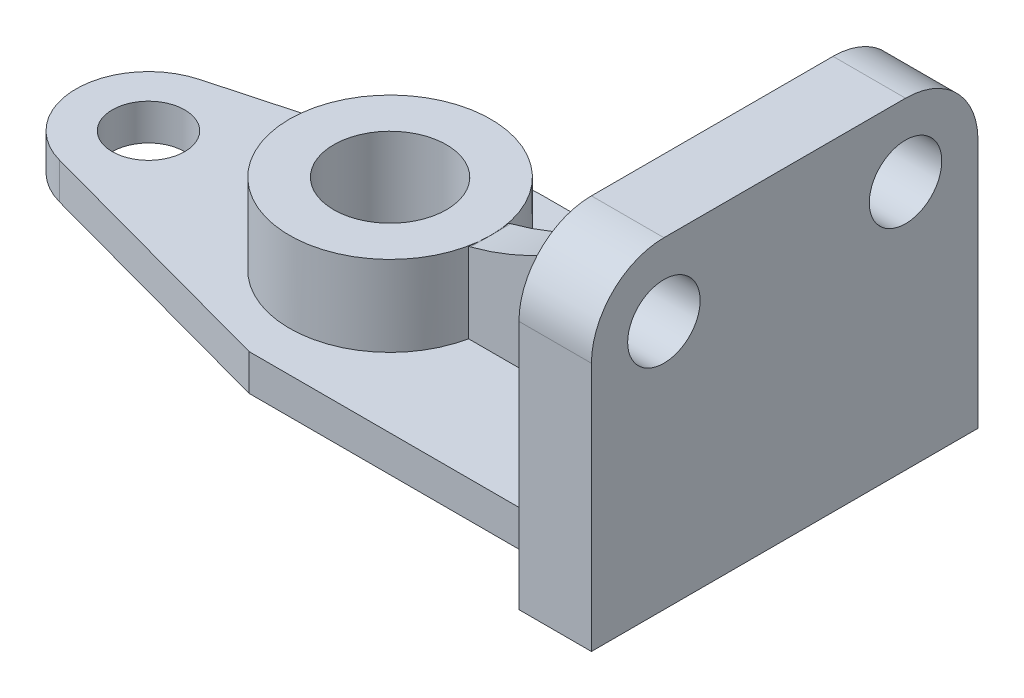
ISO-10303-21;
HEADER;
FILE_DESCRIPTION(('STEP AP214'),'2;1');
FILE_NAME('part.step','',(''),(''),'','','');
FILE_SCHEMA(('AUTOMOTIVE_DESIGN { 1 0 10303 214 1 1 1 1 }'));
ENDSEC;
DATA;
#1=APPLICATION_CONTEXT('core data for automotive mechanical design processes');
#2=APPLICATION_PROTOCOL_DEFINITION('international standard','automotive_design',2000,#1);
#3=PRODUCT_CONTEXT('',#1,'mechanical');
#4=PRODUCT('Part','Part','',(#3));
#5=PRODUCT_RELATED_PRODUCT_CATEGORY('part','',(#4));
#6=PRODUCT_DEFINITION_FORMATION('','',#4);
#7=PRODUCT_DEFINITION_CONTEXT('part definition',#1,'design');
#8=PRODUCT_DEFINITION('design','',#6,#7);
#9=PRODUCT_DEFINITION_SHAPE('','',#8);
#10=(LENGTH_UNIT() NAMED_UNIT(*) SI_UNIT(.MILLI.,.METRE.));
#11=(NAMED_UNIT(*) PLANE_ANGLE_UNIT() SI_UNIT($,.RADIAN.));
#12=(NAMED_UNIT(*) SI_UNIT($,.STERADIAN.) SOLID_ANGLE_UNIT());
#13=UNCERTAINTY_MEASURE_WITH_UNIT(LENGTH_MEASURE(1.E-05),#10,'distance_accuracy_value','');
#14=(GEOMETRIC_REPRESENTATION_CONTEXT(3) GLOBAL_UNCERTAINTY_ASSIGNED_CONTEXT((#13)) GLOBAL_UNIT_ASSIGNED_CONTEXT((#10,
#11,#12)) REPRESENTATION_CONTEXT('',''));
#15=CARTESIAN_POINT('',(0.,0.,0.));
#16=DIRECTION('',(0.,0.,1.));
#17=DIRECTION('',(1.,0.,0.));
#18=AXIS2_PLACEMENT_3D('',#15,#16,#17);
#19=CARTESIAN_POINT('',(-9.,-40.,48.));
#20=DIRECTION('',(1.,0.,0.));
#21=DIRECTION('',(0.,0.,-1.));
#22=AXIS2_PLACEMENT_3D('',#19,#20,#21);
#23=PLANE('',#22);
#24=CARTESIAN_POINT('',(-9.,22.,-30.));
#25=DIRECTION('',(-1.,0.,0.));
#26=DIRECTION('',(0.,0.,1.));
#27=AXIS2_PLACEMENT_3D('',#24,#25,#26);
#28=CIRCLE('',#27,9.);
#29=CARTESIAN_POINT('',(-9.,22.,-21.));
#30=VERTEX_POINT('',#29);
#31=EDGE_CURVE('E245',#30,#30,#28,.T.);
#32=ORIENTED_EDGE('',*,*,#31,.F.);
#33=EDGE_LOOP('',(#32));
#34=FACE_BOUND('',#33,.T.);
#35=DIRECTION('',(0.,-1.,0.));
#36=VECTOR('',#35,1.);
#37=CARTESIAN_POINT('',(-9.,-40.,-5.));
#38=LINE('',#37,#36);
#39=CARTESIAN_POINT('',(-9.,40.,-5.));
#40=VERTEX_POINT('',#39);
#41=CARTESIAN_POINT('',(-9.,-31.,-5.));
#42=VERTEX_POINT('',#41);
#43=EDGE_CURVE('E201',#40,#42,#38,.T.);
#44=ORIENTED_EDGE('',*,*,#43,.F.);
#45=DIRECTION('',(0.,0.,-1.));
#46=VECTOR('',#45,1.);
#47=CARTESIAN_POINT('',(-9.,40.,48.));
#48=LINE('',#47,#46);
#49=CARTESIAN_POINT('',(-9.,40.,-30.));
#50=VERTEX_POINT('',#49);
#51=EDGE_CURVE('E332',#40,#50,#48,.T.);
#52=ORIENTED_EDGE('',*,*,#51,.T.);
#53=CARTESIAN_POINT('',(-9.,22.,-30.));
#54=DIRECTION('',(1.,0.,0.));
#55=DIRECTION('',(0.,0.,-1.));
#56=AXIS2_PLACEMENT_3D('',#53,#54,#55);
#57=CIRCLE('',#56,18.);
#58=CARTESIAN_POINT('',(-9.,22.,-48.));
#59=VERTEX_POINT('',#58);
#60=EDGE_CURVE('E226',#50,#59,#57,.F.);
#61=ORIENTED_EDGE('',*,*,#60,.T.);
#62=DIRECTION('',(0.,-1.,0.));
#63=VECTOR('',#62,1.);
#64=CARTESIAN_POINT('',(-9.,-40.,-48.));
#65=LINE('',#64,#63);
#66=CARTESIAN_POINT('',(-9.,-31.,-48.));
#67=VERTEX_POINT('',#66);
#68=EDGE_CURVE('E326',#59,#67,#65,.T.);
#69=ORIENTED_EDGE('',*,*,#68,.T.);
#70=DIRECTION('',(0.,0.,1.));
#71=VECTOR('',#70,1.);
#72=CARTESIAN_POINT('',(-9.,-31.,-48.));
#73=LINE('',#72,#71);
#74=EDGE_CURVE('E311',#67,#42,#73,.T.);
#75=ORIENTED_EDGE('',*,*,#74,.T.);
#76=EDGE_LOOP('',(#44,#52,#61,#69,#75));
#77=FACE_BOUND('',#76,.T.);
#78=ADVANCED_FACE('F39',(#34,#77),#23,.F.);
#79=CARTESIAN_POINT('',(-9.,40.,48.));
#80=DIRECTION('',(0.,-1.,0.));
#81=DIRECTION('',(0.,0.,-1.));
#82=AXIS2_PLACEMENT_3D('',#79,#80,#81);
#83=PLANE('',#82);
#84=DIRECTION('',(0.,0.,-1.));
#85=VECTOR('',#84,1.);
#86=CARTESIAN_POINT('',(9.,40.,48.));
#87=LINE('',#86,#85);
#88=CARTESIAN_POINT('',(9.,40.,30.));
#89=VERTEX_POINT('',#88);
#90=CARTESIAN_POINT('',(9.,40.,-30.));
#91=VERTEX_POINT('',#90);
#92=EDGE_CURVE('E337',#89,#91,#87,.T.);
#93=ORIENTED_EDGE('',*,*,#92,.T.);
#94=DIRECTION('',(-1.,0.,0.));
#95=VECTOR('',#94,1.);
#96=CARTESIAN_POINT('',(9.,40.,-30.));
#97=LINE('',#96,#95);
#98=EDGE_CURVE('E231',#91,#50,#97,.T.);
#99=ORIENTED_EDGE('',*,*,#98,.T.);
#100=ORIENTED_EDGE('',*,*,#51,.F.);
#101=DIRECTION('',(0.,0.,1.));
#102=VECTOR('',#101,1.);
#103=CARTESIAN_POINT('',(-9.00000000000001,40.,0.));
#104=LINE('',#103,#102);
#105=CARTESIAN_POINT('',(-9.,40.,5.));
#106=VERTEX_POINT('',#105);
#107=EDGE_CURVE('E205',#40,#106,#104,.T.);
#108=ORIENTED_EDGE('',*,*,#107,.T.);
#109=CARTESIAN_POINT('',(-9.,40.,30.));
#110=VERTEX_POINT('',#109);
#111=EDGE_CURVE('E335',#110,#106,#48,.T.);
#112=ORIENTED_EDGE('',*,*,#111,.F.);
#113=DIRECTION('',(-1.,0.,0.));
#114=VECTOR('',#113,1.);
#115=CARTESIAN_POINT('',(9.,40.,30.));
#116=LINE('',#115,#114);
#117=EDGE_CURVE('E228',#89,#110,#116,.T.);
#118=ORIENTED_EDGE('',*,*,#117,.F.);
#119=EDGE_LOOP('',(#93,#99,#100,#108,#112,#118));
#120=FACE_BOUND('',#119,.T.);
#121=ADVANCED_FACE('F423',(#120),#83,.F.);
#122=CARTESIAN_POINT('',(0.,0.,48.));
#123=DIRECTION('',(0.,0.,-1.));
#124=DIRECTION('',(-1.,0.,0.));
#125=AXIS2_PLACEMENT_3D('',#122,#123,#124);
#126=PLANE('',#125);
#127=DIRECTION('',(-1.,0.,0.));
#128=VECTOR('',#127,1.);
#129=CARTESIAN_POINT('',(9.,22.,48.));
#130=LINE('',#129,#128);
#131=CARTESIAN_POINT('',(9.,22.,48.));
#132=VERTEX_POINT('',#131);
#133=CARTESIAN_POINT('',(-9.,22.,48.));
#134=VERTEX_POINT('',#133);
#135=EDGE_CURVE('E225',#132,#134,#130,.T.);
#136=ORIENTED_EDGE('',*,*,#135,.T.);
#137=DIRECTION('',(0.,-1.,0.));
#138=VECTOR('',#137,1.);
#139=CARTESIAN_POINT('',(-9.,-40.,48.));
#140=LINE('',#139,#138);
#141=CARTESIAN_POINT('',(-9.,-31.,48.));
#142=VERTEX_POINT('',#141);
#143=EDGE_CURVE('E316',#134,#142,#140,.T.);
#144=ORIENTED_EDGE('',*,*,#143,.T.);
#145=CARTESIAN_POINT('',(-9.00000000000001,-40.,48.));
#146=VERTEX_POINT('',#145);
#147=EDGE_CURVE('E320',#142,#146,#140,.T.);
#148=ORIENTED_EDGE('',*,*,#147,.T.);
#149=DIRECTION('',(1.,0.,0.));
#150=VECTOR('',#149,1.);
#151=CARTESIAN_POINT('',(-9.,-40.,48.));
#152=LINE('',#151,#150);
#153=CARTESIAN_POINT('',(9.,-40.,48.));
#154=VERTEX_POINT('',#153);
#155=EDGE_CURVE('E321',#146,#154,#152,.T.);
#156=ORIENTED_EDGE('',*,*,#155,.T.);
#157=DIRECTION('',(0.,1.,0.));
#158=VECTOR('',#157,1.);
#159=CARTESIAN_POINT('',(9.,-40.,48.));
#160=LINE('',#159,#158);
#161=EDGE_CURVE('E313',#154,#132,#160,.T.);
#162=ORIENTED_EDGE('',*,*,#161,.T.);
#163=EDGE_LOOP('',(#136,#144,#148,#156,#162));
#164=FACE_BOUND('',#163,.T.);
#165=ADVANCED_FACE('F429',(#164),#126,.F.);
#166=CARTESIAN_POINT('',(0.,0.,-48.));
#167=DIRECTION('',(0.,0.,-1.));
#168=DIRECTION('',(-1.,0.,0.));
#169=AXIS2_PLACEMENT_3D('',#166,#167,#168);
#170=PLANE('',#169);
#171=ORIENTED_EDGE('',*,*,#68,.F.);
#172=DIRECTION('',(-1.,0.,0.));
#173=VECTOR('',#172,1.);
#174=CARTESIAN_POINT('',(9.,22.,-48.));
#175=LINE('',#174,#173);
#176=CARTESIAN_POINT('',(9.,22.,-48.));
#177=VERTEX_POINT('',#176);
#178=EDGE_CURVE('E221',#177,#59,#175,.T.);
#179=ORIENTED_EDGE('',*,*,#178,.F.);
#180=DIRECTION('',(0.,1.,0.));
#181=VECTOR('',#180,1.);
#182=CARTESIAN_POINT('',(9.,-40.,-48.));
#183=LINE('',#182,#181);
#184=CARTESIAN_POINT('',(9.,-40.,-48.));
#185=VERTEX_POINT('',#184);
#186=EDGE_CURVE('E312',#185,#177,#183,.T.);
#187=ORIENTED_EDGE('',*,*,#186,.F.);
#188=DIRECTION('',(1.,0.,0.));
#189=VECTOR('',#188,1.);
#190=CARTESIAN_POINT('',(-9.,-40.,-48.));
#191=LINE('',#190,#189);
#192=CARTESIAN_POINT('',(-9.00000000000001,-40.,-48.));
#193=VERTEX_POINT('',#192);
#194=EDGE_CURVE('E319',#193,#185,#191,.T.);
#195=ORIENTED_EDGE('',*,*,#194,.F.);
#196=EDGE_CURVE('E330',#67,#193,#65,.T.);
#197=ORIENTED_EDGE('',*,*,#196,.F.);
#198=EDGE_LOOP('',(#171,#179,#187,#195,#197));
#199=FACE_BOUND('',#198,.T.);
#200=ADVANCED_FACE('F373',(#199),#170,.T.);
#201=CARTESIAN_POINT('',(-9.,-40.,48.));
#202=DIRECTION('',(0.,1.,0.));
#203=DIRECTION('',(0.,0.,1.));
#204=AXIS2_PLACEMENT_3D('',#201,#202,#203);
#205=PLANE('',#204);
#206=CARTESIAN_POINT('',(-149.,-40.,0.));
#207=DIRECTION('',(0.,1.,0.));
#208=DIRECTION('',(0.,0.,1.));
#209=AXIS2_PLACEMENT_3D('',#206,#207,#208);
#210=CIRCLE('',#209,9.00000000000001);
#211=CARTESIAN_POINT('',(-149.,-40.,9.00000000000001));
#212=VERTEX_POINT('',#211);
#213=EDGE_CURVE('E300',#212,#212,#210,.T.);
#214=ORIENTED_EDGE('',*,*,#213,.T.);
#215=EDGE_LOOP('',(#214));
#216=FACE_BOUND('',#215,.T.);
#217=DIRECTION('',(-0.964843429689675,0.,-0.262825333985644));
#218=VECTOR('',#217,1.);
#219=CARTESIAN_POINT('',(-15.0233522832567,-40.,55.1513909355685));
#220=LINE('',#219,#218);
#221=CARTESIAN_POINT('',(-89.,-40.,35.));
#222=VERTEX_POINT('',#221);
#223=CARTESIAN_POINT('',(-153.730856011742,-40.,17.3671817344141));
#224=VERTEX_POINT('',#223);
#225=EDGE_CURVE('E256',#222,#224,#220,.T.);
#226=ORIENTED_EDGE('',*,*,#225,.T.);
#227=CARTESIAN_POINT('',(-149.,-40.,0.));
#228=DIRECTION('',(0.,1.,0.));
#229=DIRECTION('',(0.,0.,1.));
#230=AXIS2_PLACEMENT_3D('',#227,#228,#229);
#231=CIRCLE('',#230,18.);
#232=CARTESIAN_POINT('',(-153.730856011742,-40.,-17.3671817344142));
#233=VERTEX_POINT('',#232);
#234=EDGE_CURVE('E279',#233,#224,#231,.T.);
#235=ORIENTED_EDGE('',*,*,#234,.F.);
#236=DIRECTION('',(-0.964843429689675,0.,0.262825333985644));
#237=VECTOR('',#236,1.);
#238=CARTESIAN_POINT('',(-15.0233522832567,-40.,-55.1513909355685));
#239=LINE('',#238,#237);
#240=CARTESIAN_POINT('',(-91.581226502023,-40.,-34.2968685937935));
#241=VERTEX_POINT('',#240);
#242=EDGE_CURVE('E280',#241,#233,#239,.T.);
#243=ORIENTED_EDGE('',*,*,#242,.F.);
#244=CARTESIAN_POINT('',(-86.3247198223102,-40.,-15.));
#245=DIRECTION('',(0.,1.,0.));
#246=DIRECTION('',(0.,0.,1.));
#247=AXIS2_PLACEMENT_3D('',#244,#245,#246);
#248=CIRCLE('',#247,20.);
#249=CARTESIAN_POINT('',(-86.3247198223102,-40.,-35.));
#250=VERTEX_POINT('',#249);
#251=EDGE_CURVE('E272',#250,#241,#248,.T.);
#252=ORIENTED_EDGE('',*,*,#251,.F.);
#253=DIRECTION('',(-1.,0.,0.));
#254=VECTOR('',#253,1.);
#255=CARTESIAN_POINT('',(0.,-40.,-35.));
#256=LINE('',#255,#254);
#257=CARTESIAN_POINT('',(-22.,-40.,-35.));
#258=VERTEX_POINT('',#257);
#259=EDGE_CURVE('E271',#258,#250,#256,.T.);
#260=ORIENTED_EDGE('',*,*,#259,.F.);
#261=CARTESIAN_POINT('',(-22.,-40.,-48.));
#262=DIRECTION('',(0.,1.,0.));
#263=DIRECTION('',(0.,0.,1.));
#264=AXIS2_PLACEMENT_3D('',#261,#262,#263);
#265=CIRCLE('',#264,13.);
#266=EDGE_CURVE('E11',#258,#193,#265,.T.);
#267=ORIENTED_EDGE('',*,*,#266,.T.);
#268=ORIENTED_EDGE('',*,*,#194,.T.);
#269=DIRECTION('',(0.,0.,-1.));
#270=VECTOR('',#269,1.);
#271=CARTESIAN_POINT('',(9.,-40.,48.));
#272=LINE('',#271,#270);
#273=EDGE_CURVE('E323',#154,#185,#272,.T.);
#274=ORIENTED_EDGE('',*,*,#273,.F.);
#275=ORIENTED_EDGE('',*,*,#155,.F.);
#276=CARTESIAN_POINT('',(-22.,-40.,48.));
#277=DIRECTION('',(0.,1.,0.));
#278=DIRECTION('',(0.,0.,1.));
#279=AXIS2_PLACEMENT_3D('',#276,#277,#278);
#280=CIRCLE('',#279,13.);
#281=CARTESIAN_POINT('',(-22.,-40.,35.));
#282=VERTEX_POINT('',#281);
#283=EDGE_CURVE('E350',#146,#282,#280,.T.);
#284=ORIENTED_EDGE('',*,*,#283,.T.);
#285=DIRECTION('',(-1.,0.,0.));
#286=VECTOR('',#285,1.);
#287=CARTESIAN_POINT('',(0.,-40.,35.));
#288=LINE('',#287,#286);
#289=EDGE_CURVE('E253',#282,#222,#288,.T.);
#290=ORIENTED_EDGE('',*,*,#289,.T.);
#291=EDGE_LOOP('',(#226,#235,#243,#252,#260,#267,#268,#274,#275,#284,#290));
#292=FACE_BOUND('',#291,.T.);
#293=ADVANCED_FACE('F370',(#216,#292),#205,.F.);
#294=CARTESIAN_POINT('',(-167.,-31.,-48.));
#295=DIRECTION('',(0.,1.,0.));
#296=DIRECTION('',(0.,0.,1.));
#297=AXIS2_PLACEMENT_3D('',#294,#295,#296);
#298=PLANE('',#297);
#299=DIRECTION('',(1.,0.,0.));
#300=VECTOR('',#299,1.);
#301=CARTESIAN_POINT('',(-167.,-31.,5.));
#302=LINE('',#301,#300);
#303=CARTESIAN_POINT('',(-64.5051025721682,-31.,5.));
#304=VERTEX_POINT('',#303);
#305=CARTESIAN_POINT('',(-9.,-31.,5.));
#306=VERTEX_POINT('',#305);
#307=EDGE_CURVE('E213',#304,#306,#302,.T.);
#308=ORIENTED_EDGE('',*,*,#307,.F.);
#309=CARTESIAN_POINT('',(-89.,-31.,0.));
#310=DIRECTION('',(0.,1.,0.));
#311=DIRECTION('',(0.,0.,1.));
#312=AXIS2_PLACEMENT_3D('',#309,#310,#311);
#313=CIRCLE('',#312,25.);
#314=CARTESIAN_POINT('',(-64.5051025721682,-31.,-5.));
#315=VERTEX_POINT('',#314);
#316=EDGE_CURVE('E304',#315,#304,#313,.T.);
#317=ORIENTED_EDGE('',*,*,#316,.F.);
#318=DIRECTION('',(1.,0.,0.));
#319=VECTOR('',#318,1.);
#320=CARTESIAN_POINT('',(-167.,-31.,-5.));
#321=LINE('',#320,#319);
#322=EDGE_CURVE('E61',#315,#42,#321,.T.);
#323=ORIENTED_EDGE('',*,*,#322,.T.);
#324=ORIENTED_EDGE('',*,*,#74,.F.);
#325=CARTESIAN_POINT('',(-22.,-31.,-48.));
#326=DIRECTION('',(0.,1.,0.));
#327=DIRECTION('',(0.,0.,1.));
#328=AXIS2_PLACEMENT_3D('',#325,#326,#327);
#329=CIRCLE('',#328,13.);
#330=CARTESIAN_POINT('',(-22.,-31.,-35.));
#331=VERTEX_POINT('',#330);
#332=EDGE_CURVE('E50',#67,#331,#329,.F.);
#333=ORIENTED_EDGE('',*,*,#332,.T.);
#334=DIRECTION('',(-1.,0.,0.));
#335=VECTOR('',#334,1.);
#336=CARTESIAN_POINT('',(0.,-31.,-35.));
#337=LINE('',#336,#335);
#338=CARTESIAN_POINT('',(-86.3247198223102,-31.,-35.));
#339=VERTEX_POINT('',#338);
#340=EDGE_CURVE('E281',#331,#339,#337,.T.);
#341=ORIENTED_EDGE('',*,*,#340,.T.);
#342=CARTESIAN_POINT('',(-86.3247198223102,-31.,-15.));
#343=DIRECTION('',(0.,1.,0.));
#344=DIRECTION('',(0.,0.,1.));
#345=AXIS2_PLACEMENT_3D('',#342,#343,#344);
#346=CIRCLE('',#345,20.);
#347=CARTESIAN_POINT('',(-91.581226502023,-31.,-34.2968685937935));
#348=VERTEX_POINT('',#347);
#349=EDGE_CURVE('E267',#339,#348,#346,.T.);
#350=ORIENTED_EDGE('',*,*,#349,.T.);
#351=DIRECTION('',(-0.964843429689675,0.,0.262825333985644));
#352=VECTOR('',#351,1.);
#353=CARTESIAN_POINT('',(-15.0233522832567,-31.,-55.1513909355685));
#354=LINE('',#353,#352);
#355=CARTESIAN_POINT('',(-153.730856011742,-31.,-17.3671817344142));
#356=VERTEX_POINT('',#355);
#357=EDGE_CURVE('E274',#348,#356,#354,.T.);
#358=ORIENTED_EDGE('',*,*,#357,.T.);
#359=CARTESIAN_POINT('',(-149.,-31.,0.));
#360=DIRECTION('',(0.,1.,0.));
#361=DIRECTION('',(0.,0.,1.));
#362=AXIS2_PLACEMENT_3D('',#359,#360,#361);
#363=CIRCLE('',#362,18.);
#364=CARTESIAN_POINT('',(-153.730856011742,-31.,17.3671817344141));
#365=VERTEX_POINT('',#364);
#366=EDGE_CURVE('E284',#356,#365,#363,.T.);
#367=ORIENTED_EDGE('',*,*,#366,.T.);
#368=DIRECTION('',(-0.964843429689675,0.,-0.262825333985644));
#369=VECTOR('',#368,1.);
#370=CARTESIAN_POINT('',(-15.0233522832567,-31.,55.1513909355685));
#371=LINE('',#370,#369);
#372=CARTESIAN_POINT('',(-89.,-31.,35.));
#373=VERTEX_POINT('',#372);
#374=EDGE_CURVE('E260',#373,#365,#371,.T.);
#375=ORIENTED_EDGE('',*,*,#374,.F.);
#376=DIRECTION('',(-1.,0.,0.));
#377=VECTOR('',#376,1.);
#378=CARTESIAN_POINT('',(0.,-31.,35.));
#379=LINE('',#378,#377);
#380=CARTESIAN_POINT('',(-22.,-31.,35.));
#381=VERTEX_POINT('',#380);
#382=EDGE_CURVE('E255',#381,#373,#379,.T.);
#383=ORIENTED_EDGE('',*,*,#382,.F.);
#384=CARTESIAN_POINT('',(-22.,-31.,48.));
#385=DIRECTION('',(0.,1.,0.));
#386=DIRECTION('',(0.,0.,1.));
#387=AXIS2_PLACEMENT_3D('',#384,#385,#386);
#388=CIRCLE('',#387,13.);
#389=EDGE_CURVE('E343',#381,#142,#388,.F.);
#390=ORIENTED_EDGE('',*,*,#389,.T.);
#391=EDGE_CURVE('E307',#306,#142,#73,.T.);
#392=ORIENTED_EDGE('',*,*,#391,.F.);
#393=EDGE_LOOP('',(#308,#317,#323,#324,#333,#341,#350,#358,#367,#375,#383,#390,#392));
#394=FACE_BOUND('',#393,.T.);
#395=CARTESIAN_POINT('',(-149.,-31.,0.));
#396=DIRECTION('',(0.,1.,0.));
#397=DIRECTION('',(0.,0.,1.));
#398=AXIS2_PLACEMENT_3D('',#395,#396,#397);
#399=CIRCLE('',#398,9.00000000000001);
#400=CARTESIAN_POINT('',(-149.,-31.,9.00000000000001));
#401=VERTEX_POINT('',#400);
#402=EDGE_CURVE('E292',#401,#401,#399,.T.);
#403=ORIENTED_EDGE('',*,*,#402,.F.);
#404=EDGE_LOOP('',(#403));
#405=FACE_BOUND('',#404,.T.);
#406=ADVANCED_FACE('F352',(#394,#405),#298,.T.);
#407=CARTESIAN_POINT('',(9.,-40.,48.));
#408=DIRECTION('',(-1.,0.,0.));
#409=DIRECTION('',(0.,0.,1.));
#410=AXIS2_PLACEMENT_3D('',#407,#408,#409);
#411=PLANE('',#410);
#412=CARTESIAN_POINT('',(9.,22.,30.));
#413=DIRECTION('',(-1.,0.,0.));
#414=DIRECTION('',(0.,0.,1.));
#415=AXIS2_PLACEMENT_3D('',#412,#413,#414);
#416=CIRCLE('',#415,9.);
#417=CARTESIAN_POINT('',(9.,22.,39.));
#418=VERTEX_POINT('',#417);
#419=EDGE_CURVE('E248',#418,#418,#416,.T.);
#420=ORIENTED_EDGE('',*,*,#419,.T.);
#421=EDGE_LOOP('',(#420));
#422=FACE_BOUND('',#421,.T.);
#423=ORIENTED_EDGE('',*,*,#273,.T.);
#424=ORIENTED_EDGE('',*,*,#186,.T.);
#425=CARTESIAN_POINT('',(9.,22.,-30.));
#426=DIRECTION('',(1.,0.,0.));
#427=DIRECTION('',(0.,0.,1.));
#428=AXIS2_PLACEMENT_3D('',#425,#426,#427);
#429=CIRCLE('',#428,18.);
#430=EDGE_CURVE('E219',#177,#91,#429,.T.);
#431=ORIENTED_EDGE('',*,*,#430,.T.);
#432=ORIENTED_EDGE('',*,*,#92,.F.);
#433=CARTESIAN_POINT('',(9.,22.,30.));
#434=DIRECTION('',(1.,0.,0.));
#435=DIRECTION('',(0.,0.,1.));
#436=AXIS2_PLACEMENT_3D('',#433,#434,#435);
#437=CIRCLE('',#436,18.);
#438=EDGE_CURVE('E223',#89,#132,#437,.T.);
#439=ORIENTED_EDGE('',*,*,#438,.T.);
#440=ORIENTED_EDGE('',*,*,#161,.F.);
#441=EDGE_LOOP('',(#423,#424,#431,#432,#439,#440));
#442=FACE_BOUND('',#441,.T.);
#443=CARTESIAN_POINT('',(9.,22.,-30.));
#444=DIRECTION('',(-1.,0.,0.));
#445=DIRECTION('',(0.,0.,1.));
#446=AXIS2_PLACEMENT_3D('',#443,#444,#445);
#447=CIRCLE('',#446,9.);
#448=CARTESIAN_POINT('',(9.,22.,-21.));
#449=VERTEX_POINT('',#448);
#450=EDGE_CURVE('E243',#449,#449,#447,.T.);
#451=ORIENTED_EDGE('',*,*,#450,.T.);
#452=EDGE_LOOP('',(#451));
#453=FACE_BOUND('',#452,.T.);
#454=ADVANCED_FACE('F376',(#422,#442,#453),#411,.F.);
#455=CARTESIAN_POINT('',(-9.,22.,30.));
#456=DIRECTION('',(-1.,0.,0.));
#457=DIRECTION('',(0.,0.,1.));
#458=AXIS2_PLACEMENT_3D('',#455,#456,#457);
#459=CIRCLE('',#458,9.);
#460=CARTESIAN_POINT('',(-9.,22.,39.));
#461=VERTEX_POINT('',#460);
#462=EDGE_CURVE('E246',#461,#461,#459,.T.);
#463=ORIENTED_EDGE('',*,*,#462,.F.);
#464=EDGE_LOOP('',(#463));
#465=FACE_BOUND('',#464,.T.);
#466=ORIENTED_EDGE('',*,*,#111,.T.);
#467=DIRECTION('',(0.,-1.,0.));
#468=VECTOR('',#467,1.);
#469=CARTESIAN_POINT('',(-9.,-40.,5.));
#470=LINE('',#469,#468);
#471=EDGE_CURVE('E53',#106,#306,#470,.T.);
#472=ORIENTED_EDGE('',*,*,#471,.T.);
#473=ORIENTED_EDGE('',*,*,#391,.T.);
#474=ORIENTED_EDGE('',*,*,#143,.F.);
#475=CARTESIAN_POINT('',(-9.,22.,30.));
#476=DIRECTION('',(1.,0.,0.));
#477=DIRECTION('',(0.,0.,-1.));
#478=AXIS2_PLACEMENT_3D('',#475,#476,#477);
#479=CIRCLE('',#478,18.);
#480=EDGE_CURVE('E237',#134,#110,#479,.F.);
#481=ORIENTED_EDGE('',*,*,#480,.T.);
#482=EDGE_LOOP('',(#466,#472,#473,#474,#481));
#483=FACE_BOUND('',#482,.T.);
#484=ADVANCED_FACE('F425',(#465,#483),#23,.F.);
#485=CARTESIAN_POINT('',(-89.,-11.,0.));
#486=DIRECTION('',(0.,1.,0.));
#487=DIRECTION('',(0.,0.,1.));
#488=AXIS2_PLACEMENT_3D('',#485,#486,#487);
#489=PLANE('',#488);
#490=CARTESIAN_POINT('',(-89.,-11.,0.));
#491=DIRECTION('',(0.,1.,0.));
#492=DIRECTION('',(0.,0.,1.));
#493=AXIS2_PLACEMENT_3D('',#490,#491,#492);
#494=CIRCLE('',#493,25.);
#495=CARTESIAN_POINT('',(-64.,-11.,0.));
#496=VERTEX_POINT('',#495);
#497=EDGE_CURVE('E306',#496,#496,#494,.T.);
#498=ORIENTED_EDGE('',*,*,#497,.T.);
#499=EDGE_LOOP('',(#498));
#500=FACE_BOUND('',#499,.T.);
#501=CARTESIAN_POINT('',(-89.,-11.,0.));
#502=DIRECTION('',(0.,1.,0.));
#503=DIRECTION('',(0.,0.,1.));
#504=AXIS2_PLACEMENT_3D('',#501,#502,#503);
#505=CIRCLE('',#504,14.);
#506=CARTESIAN_POINT('',(-89.,-11.,14.));
#507=VERTEX_POINT('',#506);
#508=EDGE_CURVE('E297',#507,#507,#505,.T.);
#509=ORIENTED_EDGE('',*,*,#508,.F.);
#510=EDGE_LOOP('',(#509));
#511=FACE_BOUND('',#510,.T.);
#512=ADVANCED_FACE('F436',(#500,#511),#489,.T.);
#513=CARTESIAN_POINT('',(-89.,-11.,0.));
#514=DIRECTION('',(0.,-1.,0.));
#515=DIRECTION('',(0.,0.,-1.));
#516=AXIS2_PLACEMENT_3D('',#513,#514,#515);
#517=CYLINDRICAL_SURFACE('',#516,25.);
#518=ORIENTED_EDGE('',*,*,#316,.T.);
#519=DIRECTION('',(0.,-1.,0.));
#520=VECTOR('',#519,1.);
#521=CARTESIAN_POINT('',(-64.5051025721682,-11.,5.));
#522=LINE('',#521,#520);
#523=CARTESIAN_POINT('',(-64.5051025721682,-11.1342372315239,5.));
#524=VERTEX_POINT('',#523);
#525=EDGE_CURVE('E218',#304,#524,#522,.F.);
#526=ORIENTED_EDGE('',*,*,#525,.T.);
#527=CARTESIAN_POINT('',(-89.,-17.6440580052689,0.));
#528=DIRECTION('',(-0.256846576469664,0.966452190310422,0.));
#529=DIRECTION('',(-0.966452190310422,-0.256846576469664,0.));
#530=AXIS2_PLACEMENT_3D('',#527,#528,#529);
#531=ELLIPSE('',#530,25.8678083102797,25.);
#532=EDGE_CURVE('E188',#524,#496,#531,.T.);
#533=ORIENTED_EDGE('',*,*,#532,.T.);
#534=ORIENTED_EDGE('',*,*,#497,.F.);
#535=CARTESIAN_POINT('',(-64.5051025721682,-11.1342372315239,-5.));
#536=VERTEX_POINT('',#535);
#537=EDGE_CURVE('E216',#496,#536,#531,.T.);
#538=ORIENTED_EDGE('',*,*,#537,.T.);
#539=DIRECTION('',(0.,-1.,0.));
#540=VECTOR('',#539,1.);
#541=CARTESIAN_POINT('',(-64.5051025721682,-11.,-5.));
#542=LINE('',#541,#540);
#543=EDGE_CURVE('E208',#315,#536,#542,.F.);
#544=ORIENTED_EDGE('',*,*,#543,.F.);
#545=EDGE_LOOP('',(#518,#526,#533,#534,#538,#544));
#546=FACE_BOUND('',#545,.T.);
#547=ADVANCED_FACE('F445',(#546),#517,.T.);
#548=CARTESIAN_POINT('',(-89.,-11.,0.));
#549=DIRECTION('',(0.,-1.,0.));
#550=DIRECTION('',(0.,0.,-1.));
#551=AXIS2_PLACEMENT_3D('',#548,#549,#550);
#552=CYLINDRICAL_SURFACE('',#551,14.);
#553=CARTESIAN_POINT('',(-89.,-31.,0.));
#554=DIRECTION('',(0.,1.,0.));
#555=DIRECTION('',(0.,0.,1.));
#556=AXIS2_PLACEMENT_3D('',#553,#554,#555);
#557=CIRCLE('',#556,14.);
#558=CARTESIAN_POINT('',(-89.,-31.,14.));
#559=VERTEX_POINT('',#558);
#560=EDGE_CURVE('E336',#559,#559,#557,.F.);
#561=ORIENTED_EDGE('',*,*,#560,.T.);
#562=EDGE_LOOP('',(#561));
#563=FACE_BOUND('',#562,.T.);
#564=ORIENTED_EDGE('',*,*,#508,.T.);
#565=EDGE_LOOP('',(#564));
#566=FACE_BOUND('',#565,.T.);
#567=ADVANCED_FACE('F462',(#563,#566),#552,.F.);
#568=ORIENTED_EDGE('',*,*,#560,.F.);
#569=EDGE_LOOP('',(#568));
#570=FACE_BOUND('',#569,.T.);
#571=ADVANCED_FACE('F418',(#570),#298,.T.);
#572=CARTESIAN_POINT('',(-149.,-40.,0.));
#573=DIRECTION('',(0.,1.,0.));
#574=DIRECTION('',(0.,0.,1.));
#575=AXIS2_PLACEMENT_3D('',#572,#573,#574);
#576=CYLINDRICAL_SURFACE('',#575,9.00000000000001);
#577=ORIENTED_EDGE('',*,*,#213,.F.);
#578=EDGE_LOOP('',(#577));
#579=FACE_BOUND('',#578,.T.);
#580=ORIENTED_EDGE('',*,*,#402,.T.);
#581=EDGE_LOOP('',(#580));
#582=FACE_BOUND('',#581,.T.);
#583=ADVANCED_FACE('F408',(#579,#582),#576,.F.);
#584=CARTESIAN_POINT('',(-86.3247198223102,-40.,-15.));
#585=DIRECTION('',(0.,1.,0.));
#586=DIRECTION('',(0.,0.,1.));
#587=AXIS2_PLACEMENT_3D('',#584,#585,#586);
#588=CYLINDRICAL_SURFACE('',#587,20.);
#589=ORIENTED_EDGE('',*,*,#349,.F.);
#590=DIRECTION('',(0.,1.,0.));
#591=VECTOR('',#590,1.);
#592=CARTESIAN_POINT('',(-86.3247198223102,-40.,-35.));
#593=LINE('',#592,#591);
#594=EDGE_CURVE('E277',#250,#339,#593,.T.);
#595=ORIENTED_EDGE('',*,*,#594,.F.);
#596=ORIENTED_EDGE('',*,*,#251,.T.);
#597=DIRECTION('',(0.,1.,0.));
#598=VECTOR('',#597,1.);
#599=CARTESIAN_POINT('',(-91.581226502023,-40.,-34.2968685937935));
#600=LINE('',#599,#598);
#601=EDGE_CURVE('E290',#241,#348,#600,.T.);
#602=ORIENTED_EDGE('',*,*,#601,.T.);
#603=EDGE_LOOP('',(#589,#595,#596,#602));
#604=FACE_BOUND('',#603,.T.);
#605=ADVANCED_FACE('F406',(#604),#588,.T.);
#606=CARTESIAN_POINT('',(-15.0233522832567,-40.,-55.1513909355685));
#607=DIRECTION('',(-0.262825333985644,0.,-0.964843429689675));
#608=DIRECTION('',(-0.964843429689675,0.,0.262825333985644));
#609=AXIS2_PLACEMENT_3D('',#606,#607,#608);
#610=PLANE('',#609);
#611=ORIENTED_EDGE('',*,*,#357,.F.);
#612=ORIENTED_EDGE('',*,*,#601,.F.);
#613=ORIENTED_EDGE('',*,*,#242,.T.);
#614=DIRECTION('',(0.,1.,0.));
#615=VECTOR('',#614,1.);
#616=CARTESIAN_POINT('',(-153.730856011742,-40.,-17.3671817344142));
#617=LINE('',#616,#615);
#618=EDGE_CURVE('E291',#233,#356,#617,.T.);
#619=ORIENTED_EDGE('',*,*,#618,.T.);
#620=EDGE_LOOP('',(#611,#612,#613,#619));
#621=FACE_BOUND('',#620,.T.);
#622=ADVANCED_FACE('F404',(#621),#610,.T.);
#623=CARTESIAN_POINT('',(-149.,-40.,0.));
#624=DIRECTION('',(0.,1.,0.));
#625=DIRECTION('',(0.,0.,1.));
#626=AXIS2_PLACEMENT_3D('',#623,#624,#625);
#627=CYLINDRICAL_SURFACE('',#626,18.);
#628=ORIENTED_EDGE('',*,*,#234,.T.);
#629=DIRECTION('',(0.,1.,0.));
#630=VECTOR('',#629,1.);
#631=CARTESIAN_POINT('',(-153.730856011742,-40.,17.3671817344141));
#632=LINE('',#631,#630);
#633=EDGE_CURVE('E264',#224,#365,#632,.T.);
#634=ORIENTED_EDGE('',*,*,#633,.T.);
#635=ORIENTED_EDGE('',*,*,#366,.F.);
#636=ORIENTED_EDGE('',*,*,#618,.F.);
#637=EDGE_LOOP('',(#628,#634,#635,#636));
#638=FACE_BOUND('',#637,.T.);
#639=ADVANCED_FACE('F405',(#638),#627,.T.);
#640=CARTESIAN_POINT('',(0.,-40.,-35.));
#641=DIRECTION('',(0.,0.,-1.));
#642=DIRECTION('',(-1.,0.,0.));
#643=AXIS2_PLACEMENT_3D('',#640,#641,#642);
#644=PLANE('',#643);
#645=ORIENTED_EDGE('',*,*,#340,.F.);
#646=DIRECTION('',(0.,1.,0.));
#647=VECTOR('',#646,1.);
#648=CARTESIAN_POINT('',(-22.,-40.,-35.));
#649=LINE('',#648,#647);
#650=EDGE_CURVE('E347',#331,#258,#649,.F.);
#651=ORIENTED_EDGE('',*,*,#650,.T.);
#652=ORIENTED_EDGE('',*,*,#259,.T.);
#653=ORIENTED_EDGE('',*,*,#594,.T.);
#654=EDGE_LOOP('',(#645,#651,#652,#653));
#655=FACE_BOUND('',#654,.T.);
#656=ADVANCED_FACE('F359',(#655),#644,.T.);
#657=CARTESIAN_POINT('',(-15.0233522832567,-40.,55.1513909355685));
#658=DIRECTION('',(0.262825333985644,0.,-0.964843429689675));
#659=DIRECTION('',(-0.964843429689675,0.,-0.262825333985644));
#660=AXIS2_PLACEMENT_3D('',#657,#658,#659);
#661=PLANE('',#660);
#662=ORIENTED_EDGE('',*,*,#374,.T.);
#663=ORIENTED_EDGE('',*,*,#633,.F.);
#664=ORIENTED_EDGE('',*,*,#225,.F.);
#665=DIRECTION('',(0.,1.,0.));
#666=VECTOR('',#665,1.);
#667=CARTESIAN_POINT('',(-89.,-40.,35.));
#668=LINE('',#667,#666);
#669=EDGE_CURVE('E263',#222,#373,#668,.T.);
#670=ORIENTED_EDGE('',*,*,#669,.T.);
#671=EDGE_LOOP('',(#662,#663,#664,#670));
#672=FACE_BOUND('',#671,.T.);
#673=ADVANCED_FACE('F398',(#672),#661,.F.);
#674=CARTESIAN_POINT('',(0.,-40.,35.));
#675=DIRECTION('',(0.,0.,-1.));
#676=DIRECTION('',(-1.,0.,0.));
#677=AXIS2_PLACEMENT_3D('',#674,#675,#676);
#678=PLANE('',#677);
#679=ORIENTED_EDGE('',*,*,#289,.F.);
#680=DIRECTION('',(0.,1.,0.));
#681=VECTOR('',#680,1.);
#682=CARTESIAN_POINT('',(-22.,-31.,35.));
#683=LINE('',#682,#681);
#684=EDGE_CURVE('E344',#282,#381,#683,.T.);
#685=ORIENTED_EDGE('',*,*,#684,.T.);
#686=ORIENTED_EDGE('',*,*,#382,.T.);
#687=ORIENTED_EDGE('',*,*,#669,.F.);
#688=EDGE_LOOP('',(#679,#685,#686,#687));
#689=FACE_BOUND('',#688,.T.);
#690=ADVANCED_FACE('F387',(#689),#678,.F.);
#691=CARTESIAN_POINT('',(9.,22.,30.));
#692=DIRECTION('',(-1.,0.,0.));
#693=DIRECTION('',(0.,0.,1.));
#694=AXIS2_PLACEMENT_3D('',#691,#692,#693);
#695=CYLINDRICAL_SURFACE('',#694,9.);
#696=ORIENTED_EDGE('',*,*,#419,.F.);
#697=EDGE_LOOP('',(#696));
#698=FACE_BOUND('',#697,.T.);
#699=ORIENTED_EDGE('',*,*,#462,.T.);
#700=EDGE_LOOP('',(#699));
#701=FACE_BOUND('',#700,.T.);
#702=ADVANCED_FACE('F646',(#698,#701),#695,.F.);
#703=CARTESIAN_POINT('',(-22.,-40.,48.));
#704=DIRECTION('',(0.,-1.,0.));
#705=DIRECTION('',(0.,0.,-1.));
#706=AXIS2_PLACEMENT_3D('',#703,#704,#705);
#707=CYLINDRICAL_SURFACE('',#706,13.);
#708=ORIENTED_EDGE('',*,*,#283,.F.);
#709=ORIENTED_EDGE('',*,*,#147,.F.);
#710=ORIENTED_EDGE('',*,*,#389,.F.);
#711=ORIENTED_EDGE('',*,*,#684,.F.);
#712=EDGE_LOOP('',(#708,#709,#710,#711));
#713=FACE_BOUND('',#712,.T.);
#714=ADVANCED_FACE('F386',(#713),#707,.F.);
#715=CARTESIAN_POINT('',(-22.,-40.,-48.));
#716=DIRECTION('',(0.,1.,0.));
#717=DIRECTION('',(0.,0.,1.));
#718=AXIS2_PLACEMENT_3D('',#715,#716,#717);
#719=CYLINDRICAL_SURFACE('',#718,13.);
#720=ORIENTED_EDGE('',*,*,#266,.F.);
#721=ORIENTED_EDGE('',*,*,#650,.F.);
#722=ORIENTED_EDGE('',*,*,#332,.F.);
#723=ORIENTED_EDGE('',*,*,#196,.T.);
#724=EDGE_LOOP('',(#720,#721,#722,#723));
#725=FACE_BOUND('',#724,.T.);
#726=ADVANCED_FACE('F41',(#725),#719,.F.);
#727=CARTESIAN_POINT('',(9.,22.,-30.));
#728=DIRECTION('',(-1.,0.,0.));
#729=DIRECTION('',(0.,0.,1.));
#730=AXIS2_PLACEMENT_3D('',#727,#728,#729);
#731=CYLINDRICAL_SURFACE('',#730,9.);
#732=ORIENTED_EDGE('',*,*,#450,.F.);
#733=EDGE_LOOP('',(#732));
#734=FACE_BOUND('',#733,.T.);
#735=ORIENTED_EDGE('',*,*,#31,.T.);
#736=EDGE_LOOP('',(#735));
#737=FACE_BOUND('',#736,.T.);
#738=ADVANCED_FACE('F602',(#734,#737),#731,.F.);
#739=CARTESIAN_POINT('',(9.,22.,-30.));
#740=DIRECTION('',(-1.,0.,0.));
#741=DIRECTION('',(0.,0.,1.));
#742=AXIS2_PLACEMENT_3D('',#739,#740,#741);
#743=CYLINDRICAL_SURFACE('',#742,18.);
#744=ORIENTED_EDGE('',*,*,#98,.F.);
#745=ORIENTED_EDGE('',*,*,#430,.F.);
#746=ORIENTED_EDGE('',*,*,#178,.T.);
#747=ORIENTED_EDGE('',*,*,#60,.F.);
#748=EDGE_LOOP('',(#744,#745,#746,#747));
#749=FACE_BOUND('',#748,.T.);
#750=ADVANCED_FACE('F597',(#749),#743,.T.);
#751=CARTESIAN_POINT('',(9.,22.,30.));
#752=DIRECTION('',(-1.,0.,0.));
#753=DIRECTION('',(0.,0.,1.));
#754=AXIS2_PLACEMENT_3D('',#751,#752,#753);
#755=CYLINDRICAL_SURFACE('',#754,18.);
#756=ORIENTED_EDGE('',*,*,#135,.F.);
#757=ORIENTED_EDGE('',*,*,#438,.F.);
#758=ORIENTED_EDGE('',*,*,#117,.T.);
#759=ORIENTED_EDGE('',*,*,#480,.F.);
#760=EDGE_LOOP('',(#756,#757,#758,#759));
#761=FACE_BOUND('',#760,.T.);
#762=ADVANCED_FACE('F553',(#761),#755,.T.);
#763=CARTESIAN_POINT('',(-64.,-11.,0.));
#764=DIRECTION('',(-0.256846576469664,0.966452190310422,0.));
#765=DIRECTION('',(-0.966452190310422,-0.256846576469664,0.));
#766=AXIS2_PLACEMENT_3D('',#763,#764,#765);
#767=PLANE('',#766);
#768=ORIENTED_EDGE('',*,*,#532,.F.);
#769=DIRECTION('',(-0.966452190310422,-0.256846576469664,0.));
#770=VECTOR('',#769,1.);
#771=CARTESIAN_POINT('',(-64.,-11.,5.));
#772=LINE('',#771,#770);
#773=CARTESIAN_POINT('',(-64.,-11.,5.));
#774=VERTEX_POINT('',#773);
#775=EDGE_CURVE('E189',#774,#524,#772,.T.);
#776=ORIENTED_EDGE('',*,*,#775,.F.);
#777=DIRECTION('',(0.,0.,1.));
#778=VECTOR('',#777,1.);
#779=CARTESIAN_POINT('',(-64.,-11.,0.));
#780=LINE('',#779,#778);
#781=EDGE_CURVE('E176',#496,#774,#780,.T.);
#782=ORIENTED_EDGE('',*,*,#781,.F.);
#783=EDGE_LOOP('',(#768,#776,#782));
#784=FACE_BOUND('',#783,.T.);
#785=ADVANCED_FACE('F186',(#784),#767,.T.);
#786=ORIENTED_EDGE('',*,*,#537,.F.);
#787=CARTESIAN_POINT('',(-64.,-11.,-5.));
#788=VERTEX_POINT('',#787);
#789=EDGE_CURVE('E182',#788,#496,#780,.T.);
#790=ORIENTED_EDGE('',*,*,#789,.F.);
#791=DIRECTION('',(-0.966452190310422,-0.256846576469664,0.));
#792=VECTOR('',#791,1.);
#793=CARTESIAN_POINT('',(-64.,-11.,-5.));
#794=LINE('',#793,#792);
#795=EDGE_CURVE('E203',#788,#536,#794,.T.);
#796=ORIENTED_EDGE('',*,*,#795,.T.);
#797=EDGE_LOOP('',(#786,#790,#796));
#798=FACE_BOUND('',#797,.T.);
#799=ADVANCED_FACE('F460',(#798),#767,.T.);
#800=CARTESIAN_POINT('',(-79.,0.,5.));
#801=DIRECTION('',(0.,0.,1.));
#802=DIRECTION('',(1.,0.,0.));
#803=AXIS2_PLACEMENT_3D('',#800,#801,#802);
#804=PLANE('',#803);
#805=ORIENTED_EDGE('',*,*,#525,.F.);
#806=ORIENTED_EDGE('',*,*,#307,.T.);
#807=ORIENTED_EDGE('',*,*,#471,.F.);
#808=CARTESIAN_POINT('',(-84.5477261175732,66.3161752248338,5.));
#809=DIRECTION('',(0.,0.,1.));
#810=DIRECTION('',(1.,0.,0.));
#811=AXIS2_PLACEMENT_3D('',#808,#809,#810);
#812=CIRCLE('',#811,80.);
#813=EDGE_CURVE('E181',#774,#106,#812,.T.);
#814=ORIENTED_EDGE('',*,*,#813,.F.);
#815=ORIENTED_EDGE('',*,*,#775,.T.);
#816=EDGE_LOOP('',(#805,#806,#807,#814,#815));
#817=FACE_BOUND('',#816,.T.);
#818=ADVANCED_FACE('F192',(#817),#804,.T.);
#819=CARTESIAN_POINT('',(-79.,0.,-5.));
#820=DIRECTION('',(0.,0.,1.));
#821=DIRECTION('',(1.,0.,0.));
#822=AXIS2_PLACEMENT_3D('',#819,#820,#821);
#823=PLANE('',#822);
#824=ORIENTED_EDGE('',*,*,#322,.F.);
#825=ORIENTED_EDGE('',*,*,#543,.T.);
#826=ORIENTED_EDGE('',*,*,#795,.F.);
#827=CARTESIAN_POINT('',(-84.5477261175732,66.3161752248338,-5.));
#828=DIRECTION('',(0.,0.,1.));
#829=DIRECTION('',(1.,0.,0.));
#830=AXIS2_PLACEMENT_3D('',#827,#828,#829);
#831=CIRCLE('',#830,80.);
#832=EDGE_CURVE('E195',#788,#40,#831,.T.);
#833=ORIENTED_EDGE('',*,*,#832,.T.);
#834=ORIENTED_EDGE('',*,*,#43,.T.);
#835=EDGE_LOOP('',(#824,#825,#826,#833,#834));
#836=FACE_BOUND('',#835,.T.);
#837=ADVANCED_FACE('F453',(#836),#823,.F.);
#838=CARTESIAN_POINT('',(-84.5477261175732,66.3161752248338,0.));
#839=DIRECTION('',(0.,0.,1.));
#840=DIRECTION('',(1.,0.,0.));
#841=AXIS2_PLACEMENT_3D('',#838,#839,#840);
#842=CYLINDRICAL_SURFACE('',#841,80.);
#843=ORIENTED_EDGE('',*,*,#107,.F.);
#844=ORIENTED_EDGE('',*,*,#832,.F.);
#845=ORIENTED_EDGE('',*,*,#789,.T.);
#846=ORIENTED_EDGE('',*,*,#781,.T.);
#847=ORIENTED_EDGE('',*,*,#813,.T.);
#848=EDGE_LOOP('',(#843,#844,#845,#846,#847));
#849=FACE_BOUND('',#848,.T.);
#850=ADVANCED_FACE('F177',(#849),#842,.F.);
#851=CLOSED_SHELL('',(#78,#121,#165,#200,#293,#406,#454,#484,#512,#547,#567,#571,#583,#605,#622,
#639,#656,#673,#690,#702,#714,#726,#738,#750,#762,#785,#799,#818,#837,#850));
#852=MANIFOLD_SOLID_BREP('B2',#851);
#853=ADVANCED_BREP_SHAPE_REPRESENTATION('',(#18,#852),#14);
#854=SHAPE_DEFINITION_REPRESENTATION(#9,#853);
ENDSEC;
END-ISO-10303-21;
